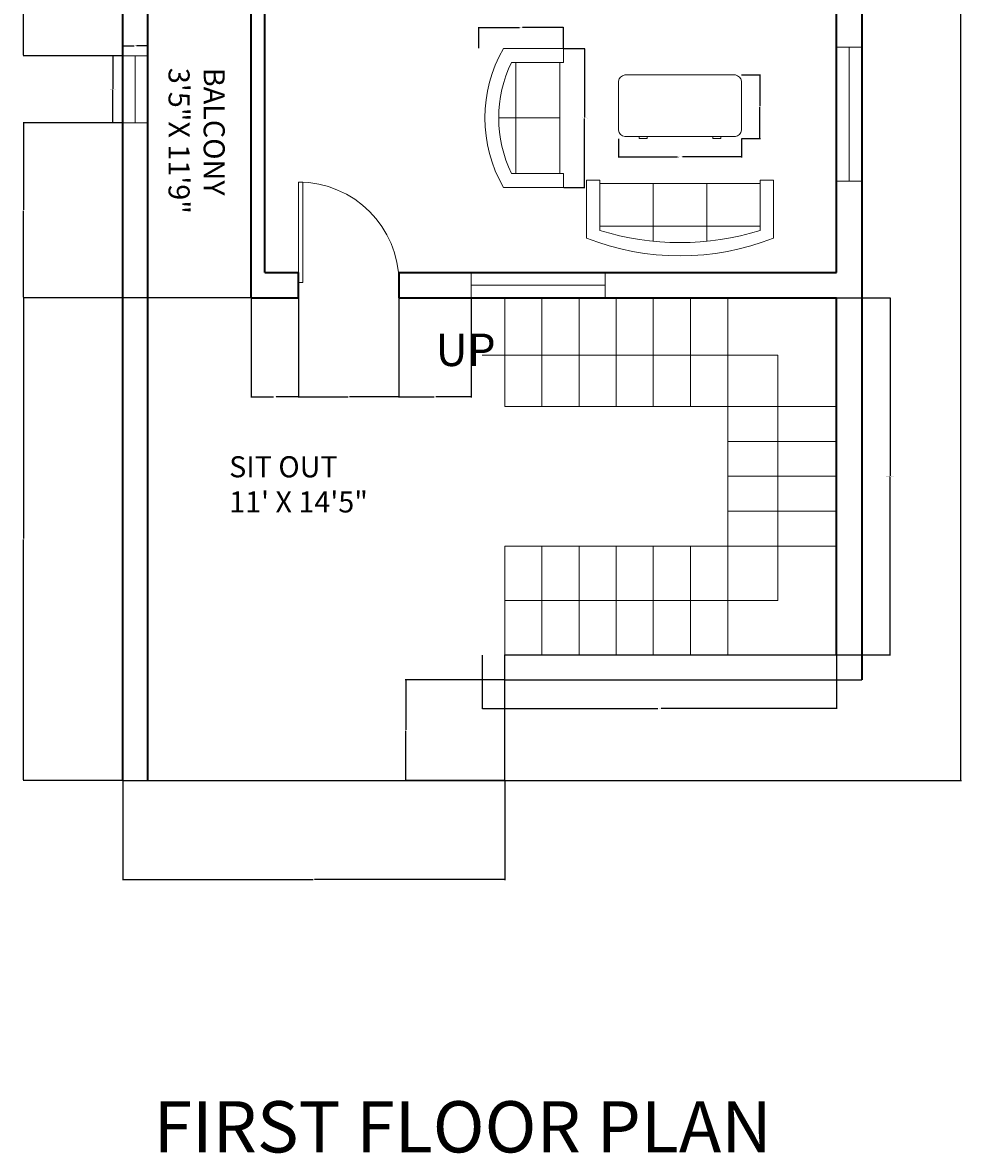
# Model space of a CAD drawing. Units: inches. Extents: x 7766 to 8631, y 9203 to 9940.
# Tile 5 of 6: x 8294 to 8631, y 9203 to 9608. Entities that reach past the tile are written whole.
import ezdxf

# ---------------------------------------------------------------- set-up
doc = ezdxf.new("R2010")
doc.units = ezdxf.units.IN
for name, color, linetype, lineweight in [('A-ANNO-DIMS', 2, 'Continuous', 18), ('A-ANNO-TEXT', 7, 'Continuous', 18), ('A-AREA-IDEN', 11, 'Continuous', 18), ('A-WALL', 7, 'Continuous', 35), ('door', 1, 'Continuous', 18), ('floor', 7, 'Continuous', 25), ('furniture', 6, 'Continuous', 18), ('stair', 2, 'Continuous', 18), ('TITLE', 4, 'Continuous', 35), ('window', 3, 'Continuous', 18)]:
    doc.layers.add(name, color=color, linetype=linetype, lineweight=lineweight)
doc.styles.get("Standard").update_dxf_attribs({"font": 'arial.ttf'})
doc.dimstyles.get("Standard").update_dxf_attribs({"dimtxt": 0.18, "dimasz": 0.18, "dimexe": 0.18, "dimexo": 0.0625, "dimgap": 0.09, "dimtad": 0, "dimtih": 1, "dimtoh": 1, "dimdec": 4, "dimzin": 0, "dimdsep": 46, "dimtxsty": 'Standard', "dimcen": 0.09, "dimadec": 0, "dimazin": 0, "dimtfac": 1, "dimtdec": 4, "dimtofl": 0, "dimtmove": 0, "dimatfit": 3, "dimfxl": 1, "dimtolj": 1, "dimtzin": 0, "dimarcsym": 0})

# ---------------------------------------------------------------- blocks, each defined once
blk = doc.blocks.new('*U2')
for p, q in [((0, 0), (0, -6)), ((40, 0), (40, -6))]:
    blk.add_line(p, q)
blk.add_lwpolyline([(0, 0), (0, 40), (1.75, 40), (1.75, 0)], close=True)
blk.add_arc((0, 0), 40, 0, 90)
blk = doc.blocks.new('Desk - 30 x 60 in.')
for p, q in [((-26.999995, 0), (26.999995, 0)), ((-29.999995, -27), (-29.999995, -3)), ((29.999995, -3), (29.999995, -27)), ((26.999995, -30), (-26.999995, -30)), ((-20.000005, -30), (-20.000005, -31)), ((-20.000005, -31), (-16.000005, -31)), ((-16.000005, -31), (-16.000005, -30)), ((15.999995, -31), (15.999995, -30)), ((19.999995, -31), (15.999995, -31)), ((19.999995, -30), (19.999995, -31))]:
    blk.add_line(p, q)
for centre, start, end in [((-26.499995, -3.5), 98.1301, 171.8699), ((26.499995, -3.5), 8.130102, 81.8699), ((-26.499995, -26.5), 188.1301, 261.8699), ((26.499995, -26.5), 278.1301, 351.8699)]:
    blk.add_arc(centre, 3.535534, start, end)
blk = doc.blocks.new('Sofa - Roundback Loveseat 5 ft.')
for p, q in [((0, -32.44198), (0, -5.99998)), ((-24, -33.99998), (-24, -11.46958)), ((-23.9998, -13.38178), (23.99986, -13.38178)), ((24.00004, -33.99998), (24.00004, -11.46958)), ((-24, -32.44198), (24.00004, -32.44198))]:
    blk.add_line(p, q)
for points in [[(-24, -33.99998), (-30, -33.99998), (-30, -7.99998)], [(30.00004, -7.99998), (30.00004, -33.99998), (24.00004, -33.99998)]]:
    blk.add_lwpolyline(points)
for centre, radius, start, end in [((0, -60.24998), 60.24998, 60.13715, 119.8628), ((0, -61.38438), 55.38444, 64.32083, 115.6792)]:
    blk.add_arc(centre, radius, start, end)
blk = doc.blocks.new('Sofa - Roundback 7 ft.')
for p, q in [((-12.00002, -32.4421), (-12.00003, -6.5971)), ((11.99997, -32.4421), (11.99998, -6.5971)), ((-36.000027, -34), (-36.000027, -11.4696)), ((-35.999844, -13.3819), (35.9998, -13.3819)), ((35.99998, -34), (35.99998, -11.4696)), ((-36.000027, -32.4421), (35.99998, -32.4421))]:
    blk.add_line(p, q)
for points in [[(-36.000027, -34), (-42.000027, -34), (-42.000027, -8)], [(41.99998, -8), (41.99998, -34), (35.99998, -34)]]:
    blk.add_lwpolyline(points)
for centre, radius, start, end in [((0, -114.25), 114.25, 68.43141, 111.5686), ((-0.00001, -127.1968), 121.1968, 72.72033, 107.2797)]:
    blk.add_arc(centre, radius, start, end)
blk = doc.blocks.new('WIN-48IN')
blk.add_line((4.5, 48), (4.5, 0))
blk.add_lwpolyline([(0, 48), (9, 48), (9, 0), (0, 0)], close=True)
blk = doc.blocks.new('WIN-24IN')
blk.add_line((4.5, 24), (4.5, 0))
blk.add_lwpolyline([(0, 24), (9, 24), (9, 0), (0, 0)], close=True)
blk = doc.blocks.new('STAIR-U-RETURN')
for p, q in [((8.13, 89), (8.13, 128)), ((21.45, 89), (21.45, 128)), ((34.76, 89), (34.76, 128)), ((48.08, 89), (48.08, 128)), ((61.39, 89), (61.39, 128)), ((74.71, 89), (74.71, 128)), ((88.13, 0), (88.13, 128)), ((0, 107.36), (106.07, 107.36)), ((106.07, 107.36), (106.07, 19.51)), ((13.13, 89), (8.13, 89)), ((13.13, 89), (88.13, 89)), ((88.13, 89), (127.13, 89)), ((88.13, 76.5), (127.13, 76.5)), ((88.13, 64), (127.13, 64)), ((88.13, 51.5), (127.13, 51.5)), ((8.13, 39), (88.13, 39)), ((8.13, 39), (8.13, 0)), ((21.45, 39), (21.45, 0)), ((34.76, 39), (34.76, 0)), ((48.08, 39), (48.08, 0)), ((61.39, 39), (61.39, 0)), ((74.71, 39), (74.71, 0)), ((88.13, 39), (127.13, 39)), ((106.07, 19.51), (8.13, 19.5))]:
    blk.add_line(p, q)
blk = doc.blocks.new('*D30')
at = {"layer": 'A-ANNO-DIMS', "color": 0, "lineweight": -2, "transparency": 16777216}
for p, q in [((8329.77, 9596.24), (8326.06, 9596.24)), ((8326.24, 9596.06), (8326.24, 9584.42)), ((8326.24, 9572.42), (8326.24, 9584.05)), ((8329.77, 9572.24), (8326.06, 9572.24))]:
    blk.add_line(p, q, dxfattribs=at)
at = {"layer": 'A-ANNO-DIMS', "color": 0, "transparency": 16777216}
for points in [[(8326.21, 9596.06), (8326.27, 9596.06), (8326.24, 9596.24)], [(8326.21, 9572.42), (8326.27, 9572.42), (8326.24, 9572.24)]]:
    blk.add_solid(points, dxfattribs=at)
at = {"layer": 'Defpoints', "color": 0, "transparency": 16777216}
for p in [(8326.24, 9596.24), (8329.84, 9596.24), (8329.84, 9572.24)]:
    blk.add_point(p, dxfattribs=at)
at = {"layer": 'A-ANNO-DIMS', "color": 0, "transparency": 16777216, "insert": (8326.24, 9584.24), "char_height": 0.18, "attachment_point": 5}
blk.add_mtext('\\A1;WINDOW 24 TYP.', dxfattribs=at)
blk = doc.blocks.new('*D31')
at = {"layer": 'A-ANNO-DIMS', "color": 0, "lineweight": -2, "transparency": 16777216}
for p, q in [((8329.84, 9596.3), (8329.84, 9600.02)), ((8330.02, 9599.84), (8333.88, 9599.84)), ((8338.66, 9599.84), (8334.79, 9599.84)), ((8338.84, 9596.3), (8338.84, 9600.02))]:
    blk.add_line(p, q, dxfattribs=at)
at = {"layer": 'A-ANNO-DIMS', "color": 0, "transparency": 16777216}
for points in [[(8330.02, 9599.87), (8330.02, 9599.81), (8329.84, 9599.84)], [(8338.66, 9599.87), (8338.66, 9599.81), (8338.84, 9599.84)]]:
    blk.add_solid(points, dxfattribs=at)
at = {"layer": 'Defpoints', "color": 0, "transparency": 16777216}
for p in [(8338.84, 9599.84), (8329.84, 9596.24), (8338.84, 9596.24)]:
    blk.add_point(p, dxfattribs=at)
at = {"layer": 'A-ANNO-DIMS', "color": 0, "transparency": 16777216, "insert": (8334.34, 9599.84), "char_height": 0.18, "attachment_point": 5}
blk.add_mtext('\\A1;9 TYP.', dxfattribs=at)
blk = doc.blocks.new('*D40')
at = {"layer": 'A-ANNO-DIMS', "color": 0, "lineweight": -2, "transparency": 16777216}
for p, q in [((8507.64, 9566.53), (8507.64, 9559.8)), ((8551.72, 9566.53), (8551.72, 9559.8)), ((8507.82, 9559.98), (8528.78, 9559.98)), ((8551.54, 9559.98), (8530.58, 9559.98))]:
    blk.add_line(p, q, dxfattribs=at)
at = {"layer": 'A-ANNO-DIMS', "color": 0, "transparency": 16777216}
for points in [[(8507.82, 9560.01), (8507.82, 9559.95), (8507.64, 9559.98)], [(8551.54, 9560.01), (8551.54, 9559.95), (8551.72, 9559.98)]]:
    blk.add_solid(points, dxfattribs=at)
at = {"layer": 'Defpoints', "color": 0, "transparency": 16777216}
for p in [(8507.64, 9566.59), (8551.72, 9566.59), (8551.72, 9559.98)]:
    blk.add_point(p, dxfattribs=at)
at = {"layer": 'A-ANNO-DIMS', "color": 0, "transparency": 16777216, "insert": (8529.68, 9559.98), "char_height": 0.18, "attachment_point": 5}
blk.add_mtext('\\A1;DESK 44 TYP.', dxfattribs=at)
blk = doc.blocks.new('*D41')
at = {"layer": 'A-ANNO-DIMS', "color": 0, "lineweight": -2, "transparency": 16777216}
for p, q in [((8551.78, 9589.37), (8558.51, 9589.37)), ((8558.33, 9589.19), (8558.33, 9578.16)), ((8558.33, 9566.77), (8558.33, 9577.8)), ((8551.78, 9566.59), (8558.51, 9566.59))]:
    blk.add_line(p, q, dxfattribs=at)
at = {"layer": 'A-ANNO-DIMS', "color": 0, "transparency": 16777216}
for points in [[(8558.3, 9589.19), (8558.36, 9589.19), (8558.33, 9589.37)], [(8558.3, 9566.77), (8558.36, 9566.77), (8558.33, 9566.59)]]:
    blk.add_solid(points, dxfattribs=at)
at = {"layer": 'Defpoints', "color": 0, "transparency": 16777216}
for p in [(8551.72, 9589.37), (8558.33, 9589.37), (8551.72, 9566.59)]:
    blk.add_point(p, dxfattribs=at)
at = {"layer": 'A-ANNO-DIMS', "color": 0, "transparency": 16777216, "insert": (8558.33, 9577.98), "char_height": 0.18, "attachment_point": 5}
blk.add_mtext('\\A1;23 TYP.', dxfattribs=at)
blk = doc.blocks.new('*D42')
at = {"layer": 'A-ANNO-DIMS', "color": 0, "lineweight": -2, "transparency": 16777216}
for p, q in [((8487.98, 9598.87), (8495.56, 9598.87)), ((8495.38, 9598.69), (8495.38, 9574.16)), ((8495.38, 9549.27), (8495.38, 9573.8)), ((8487.98, 9549.09), (8495.56, 9549.09))]:
    blk.add_line(p, q, dxfattribs=at)
at = {"layer": 'A-ANNO-DIMS', "color": 0, "transparency": 16777216}
for points in [[(8495.35, 9598.69), (8495.41, 9598.69), (8495.38, 9598.87)], [(8495.35, 9549.27), (8495.41, 9549.27), (8495.38, 9549.09)]]:
    blk.add_solid(points, dxfattribs=at)
at = {"layer": 'Defpoints', "color": 0, "transparency": 16777216}
for p in [(8487.91, 9598.87), (8495.38, 9598.87), (8487.91, 9549.09)]:
    blk.add_point(p, dxfattribs=at)
at = {"layer": 'A-ANNO-DIMS', "color": 0, "transparency": 16777216, "insert": (8495.38, 9573.98), "char_height": 0.18, "attachment_point": 5}
blk.add_mtext('\\A1;LOVESEAT 50 TYP.', dxfattribs=at)
blk = doc.blocks.new('*D43')
at = {"layer": 'A-ANNO-DIMS', "color": 0, "lineweight": -2, "transparency": 16777216}
for p, q in [((8457.49, 9598.93), (8457.49, 9606.52)), ((8457.67, 9606.34), (8472.17, 9606.34)), ((8487.73, 9606.34), (8473.23, 9606.34)), ((8487.91, 9598.93), (8487.91, 9606.52))]:
    blk.add_line(p, q, dxfattribs=at)
at = {"layer": 'A-ANNO-DIMS', "color": 0, "transparency": 16777216}
for points in [[(8457.67, 9606.37), (8457.67, 9606.31), (8457.49, 9606.34)], [(8487.73, 9606.37), (8487.73, 9606.31), (8487.91, 9606.34)]]:
    blk.add_solid(points, dxfattribs=at)
at = {"layer": 'Defpoints', "color": 0, "transparency": 16777216}
for p in [(8457.49, 9606.34), (8457.49, 9598.87), (8487.91, 9598.87)]:
    blk.add_point(p, dxfattribs=at)
at = {"layer": 'A-ANNO-DIMS', "color": 0, "transparency": 16777216, "insert": (8472.7, 9606.34), "char_height": 0.18, "attachment_point": 5}
blk.add_mtext('\\A1;30 TYP.', dxfattribs=at)
blk = doc.blocks.new('*D60')
at = {"layer": 'A-ANNO-DIMS', "color": 0, "lineweight": -2, "transparency": 16777216}
for p, q in [((8585.9, 9509.56), (8605.22, 9509.56)), ((8605.04, 9509.38), (8605.04, 9445.75)), ((8605.04, 9381.74), (8605.04, 9445.38)), ((8585.9, 9381.56), (8605.22, 9381.56))]:
    blk.add_line(p, q, dxfattribs=at)
at = {"layer": 'A-ANNO-DIMS', "color": 0, "transparency": 16777216}
for points in [[(8605.01, 9509.38), (8605.07, 9509.38), (8605.04, 9509.56)], [(8605.01, 9381.74), (8605.07, 9381.74), (8605.04, 9381.56)]]:
    blk.add_solid(points, dxfattribs=at)
at = {"layer": 'Defpoints', "color": 0, "transparency": 16777216}
for p in [(8585.84, 9509.56), (8605.04, 9509.56), (8585.84, 9381.56)]:
    blk.add_point(p, dxfattribs=at)
at = {"layer": 'A-ANNO-DIMS', "color": 0, "transparency": 16777216, "insert": (8605.04, 9445.56), "char_height": 0.18, "attachment_point": 5}
blk.add_mtext('\\A1;RETURN STAIR 128 TYP.', dxfattribs=at)
blk = doc.blocks.new('*D61')
at = {"layer": 'A-ANNO-DIMS', "color": 0, "lineweight": -2, "transparency": 16777216}
for p, q in [((8458.7, 9381.5), (8458.7, 9362.18)), ((8585.84, 9381.5), (8585.84, 9362.18)), ((8458.88, 9362.36), (8521.68, 9362.36)), ((8585.66, 9362.36), (8522.86, 9362.36))]:
    blk.add_line(p, q, dxfattribs=at)
at = {"layer": 'A-ANNO-DIMS', "color": 0, "transparency": 16777216}
for points in [[(8458.88, 9362.39), (8458.88, 9362.33), (8458.7, 9362.36)], [(8585.66, 9362.39), (8585.66, 9362.33), (8585.84, 9362.36)]]:
    blk.add_solid(points, dxfattribs=at)
at = {"layer": 'Defpoints', "color": 0, "transparency": 16777216}
for p in [(8458.7, 9381.56), (8585.84, 9381.56), (8585.84, 9362.36)]:
    blk.add_point(p, dxfattribs=at)
at = {"layer": 'A-ANNO-DIMS', "color": 0, "transparency": 16777216, "insert": (8522.27, 9362.36), "char_height": 0.18, "attachment_point": 5}
blk.add_mtext('\\A1;127 TYP.', dxfattribs=at)
blk = doc.blocks.new('*D71')
at = {"layer": 'A-ANNO-DIMS', "color": 0, "lineweight": -2, "transparency": 16777216}
for p, q in [((8594.9, 9904.56), (8630.57, 9904.56)), ((8630.39, 9904.38), (8630.39, 9620.75)), ((8630.39, 9336.74), (8630.39, 9620.38)), ((8466.9, 9336.56), (8630.57, 9336.56))]:
    blk.add_line(p, q, dxfattribs=at)
at = {"layer": 'A-ANNO-DIMS', "color": 0, "transparency": 16777216}
for points in [[(8630.36, 9904.38), (8630.42, 9904.38), (8630.39, 9904.56)], [(8630.36, 9336.74), (8630.42, 9336.74), (8630.39, 9336.56)]]:
    blk.add_solid(points, dxfattribs=at)
at = {"layer": 'Defpoints', "color": 0, "transparency": 16777216}
for p in [(8594.84, 9904.56), (8630.39, 9904.56), (8466.84, 9336.56)]:
    blk.add_point(p, dxfattribs=at)
at = {"layer": 'A-ANNO-DIMS', "color": 0, "transparency": 16777216, "insert": (8630.39, 9620.56), "char_height": 0.18, "attachment_point": 5}
blk.add_mtext('\\A1;568', dxfattribs=at)
blk = doc.blocks.new('*D73')
at = {"layer": 'A-ANNO-DIMS', "color": 0, "lineweight": -2, "transparency": 16777216}
for p, q in [((8329.84, 9336.5), (8329.84, 9300.83)), ((8466.84, 9336.5), (8466.84, 9300.83)), ((8330.02, 9301.01), (8398.06, 9301.01)), ((8466.66, 9301.01), (8398.62, 9301.01))]:
    blk.add_line(p, q, dxfattribs=at)
at = {"layer": 'A-ANNO-DIMS', "color": 0, "transparency": 16777216}
for points in [[(8330.02, 9301.04), (8330.02, 9300.98), (8329.84, 9301.01)], [(8466.66, 9301.04), (8466.66, 9300.98), (8466.84, 9301.01)]]:
    blk.add_solid(points, dxfattribs=at)
at = {"layer": 'Defpoints', "color": 0, "transparency": 16777216}
for p in [(8329.84, 9336.56), (8466.84, 9336.56), (8466.84, 9301.01)]:
    blk.add_point(p, dxfattribs=at)
at = {"layer": 'A-ANNO-DIMS', "color": 0, "transparency": 16777216, "insert": (8398.34, 9301.01), "char_height": 0.18, "attachment_point": 5}
blk.add_mtext('\\A1;137', dxfattribs=at)
blk = doc.blocks.new('*D74')
at = {"layer": 'A-ANNO-DIMS', "color": 0, "lineweight": -2, "transparency": 16777216}
for p, q in [((8375.77, 9509.56), (8294.11, 9509.56)), ((8294.29, 9509.38), (8294.29, 9423.25)), ((8294.29, 9336.74), (8294.29, 9422.88)), ((8329.77, 9336.56), (8294.11, 9336.56))]:
    blk.add_line(p, q, dxfattribs=at)
at = {"layer": 'A-ANNO-DIMS', "color": 0, "transparency": 16777216}
for points in [[(8294.26, 9509.38), (8294.32, 9509.38), (8294.29, 9509.56)], [(8294.26, 9336.74), (8294.32, 9336.74), (8294.29, 9336.56)]]:
    blk.add_solid(points, dxfattribs=at)
at = {"layer": 'Defpoints', "color": 0, "transparency": 16777216}
for p in [(8294.29, 9509.56), (8375.84, 9509.56), (8329.84, 9336.56)]:
    blk.add_point(p, dxfattribs=at)
at = {"layer": 'A-ANNO-DIMS', "color": 0, "transparency": 16777216, "insert": (8294.29, 9423.06), "char_height": 0.18, "attachment_point": 5}
blk.add_mtext('\\A1;173', dxfattribs=at)
blk = doc.blocks.new('*D75')
at = {"layer": 'A-ANNO-DIMS', "color": 0, "lineweight": -2, "transparency": 16777216}
for p, q in [((8466.77, 9372.56), (8431.11, 9372.56)), ((8431.29, 9372.38), (8431.29, 9354.75)), ((8431.29, 9336.74), (8431.29, 9354.38)), ((8466.77, 9336.56), (8431.11, 9336.56))]:
    blk.add_line(p, q, dxfattribs=at)
at = {"layer": 'A-ANNO-DIMS', "color": 0, "transparency": 16777216}
for points in [[(8431.26, 9372.38), (8431.32, 9372.38), (8431.29, 9372.56)], [(8431.26, 9336.74), (8431.32, 9336.74), (8431.29, 9336.56)]]:
    blk.add_solid(points, dxfattribs=at)
at = {"layer": 'Defpoints', "color": 0, "transparency": 16777216}
for p in [(8431.29, 9372.56), (8466.84, 9372.56), (8466.84, 9336.56)]:
    blk.add_point(p, dxfattribs=at)
at = {"layer": 'A-ANNO-DIMS', "color": 0, "transparency": 16777216, "insert": (8431.29, 9354.56), "char_height": 0.18, "attachment_point": 5}
blk.add_mtext('\\A1;36', dxfattribs=at)
blk = doc.blocks.new('*D79')
at = {"layer": 'A-ANNO-DIMS', "color": 0, "lineweight": -2, "transparency": 16777216}
for p, q in [((8329.77, 9698.92), (8294.11, 9698.92)), ((8294.29, 9698.74), (8294.29, 9647.76)), ((8294.29, 9596.42), (8294.29, 9647.4)), ((8329.77, 9596.24), (8294.11, 9596.24))]:
    blk.add_line(p, q, dxfattribs=at)
at = {"layer": 'A-ANNO-DIMS', "color": 0, "transparency": 16777216}
for points in [[(8294.26, 9698.74), (8294.32, 9698.74), (8294.29, 9698.92)], [(8294.26, 9596.42), (8294.32, 9596.42), (8294.29, 9596.24)]]:
    blk.add_solid(points, dxfattribs=at)
at = {"layer": 'Defpoints', "color": 0, "transparency": 16777216}
for p in [(8294.29, 9698.92), (8329.84, 9698.92), (8329.84, 9596.24)]:
    blk.add_point(p, dxfattribs=at)
at = {"layer": 'A-ANNO-DIMS', "color": 0, "transparency": 16777216, "insert": (8294.29, 9647.58), "char_height": 0.18, "attachment_point": 5}
blk.add_mtext('\\A1;102.69', dxfattribs=at)
blk = doc.blocks.new('*D80')
at = {"layer": 'A-ANNO-DIMS', "color": 0, "lineweight": -2, "transparency": 16777216}
for p, q in [((8329.77, 9572.24), (8294.11, 9572.24)), ((8294.29, 9572.06), (8294.29, 9541.08)), ((8294.29, 9509.74), (8294.29, 9540.72)), ((8375.77, 9509.56), (8294.11, 9509.56))]:
    blk.add_line(p, q, dxfattribs=at)
at = {"layer": 'A-ANNO-DIMS', "color": 0, "transparency": 16777216}
for points in [[(8294.26, 9572.06), (8294.32, 9572.06), (8294.29, 9572.24)], [(8294.26, 9509.74), (8294.32, 9509.74), (8294.29, 9509.56)]]:
    blk.add_solid(points, dxfattribs=at)
at = {"layer": 'Defpoints', "color": 0, "transparency": 16777216}
for p in [(8294.29, 9572.24), (8329.84, 9572.24), (8375.84, 9509.56)]:
    blk.add_point(p, dxfattribs=at)
at = {"layer": 'A-ANNO-DIMS', "color": 0, "transparency": 16777216, "insert": (8294.29, 9540.9), "char_height": 0.18, "attachment_point": 5}
blk.add_mtext('\\A1;62.67', dxfattribs=at)
blk = doc.blocks.new('*D87')
at = {"layer": 'A-ANNO-DIMS', "color": 0, "lineweight": -2, "transparency": 16777216}
for p, q in [((8392.89, 9509.5), (8392.89, 9473.83)), ((8428.89, 9509.5), (8428.89, 9473.83)), ((8393.07, 9474.01), (8410.67, 9474.01)), ((8428.71, 9474.01), (8411.11, 9474.01))]:
    blk.add_line(p, q, dxfattribs=at)
at = {"layer": 'A-ANNO-DIMS', "color": 0, "transparency": 16777216}
for points in [[(8393.07, 9474.04), (8393.07, 9473.98), (8392.89, 9474.01)], [(8428.71, 9474.04), (8428.71, 9473.98), (8428.89, 9474.01)]]:
    blk.add_solid(points, dxfattribs=at)
at = {"layer": 'Defpoints', "color": 0, "transparency": 16777216}
for p in [(8392.89, 9509.56), (8428.89, 9509.56), (8392.89, 9474.01)]:
    blk.add_point(p, dxfattribs=at)
at = {"layer": 'A-ANNO-DIMS', "color": 0, "transparency": 16777216, "insert": (8410.89, 9474.01), "char_height": 0.18, "attachment_point": 5}
blk.add_mtext('\\A1;36', dxfattribs=at)
blk = doc.blocks.new('*D88')
at = {"layer": 'A-ANNO-DIMS', "color": 0, "lineweight": -2, "transparency": 16777216}
for p, q in [((8428.89, 9509.5), (8428.89, 9473.83)), ((8454.79, 9509.5), (8454.79, 9473.83)), ((8429.07, 9474.01), (8441.51, 9474.01)), ((8454.61, 9474.01), (8442.16, 9474.01))]:
    blk.add_line(p, q, dxfattribs=at)
at = {"layer": 'A-ANNO-DIMS', "color": 0, "transparency": 16777216}
for points in [[(8429.07, 9474.04), (8429.07, 9473.98), (8428.89, 9474.01)], [(8454.61, 9474.04), (8454.61, 9473.98), (8454.79, 9474.01)]]:
    blk.add_solid(points, dxfattribs=at)
at = {"layer": 'Defpoints', "color": 0, "transparency": 16777216}
for p in [(8428.89, 9509.56), (8454.79, 9509.56), (8428.89, 9474.01)]:
    blk.add_point(p, dxfattribs=at)
at = {"layer": 'A-ANNO-DIMS', "color": 0, "transparency": 16777216, "insert": (8441.84, 9474.01), "char_height": 0.18, "attachment_point": 5}
blk.add_mtext('\\A1;25.9', dxfattribs=at)
blk = doc.blocks.new('*D89')
at = {"layer": 'A-ANNO-DIMS', "color": 0, "lineweight": -2, "transparency": 16777216}
for p, q in [((8375.84, 9509.5), (8375.84, 9473.83)), ((8392.89, 9509.5), (8392.89, 9473.83)), ((8376.02, 9474.01), (8383.91, 9474.01)), ((8392.71, 9474.01), (8384.82, 9474.01))]:
    blk.add_line(p, q, dxfattribs=at)
at = {"layer": 'A-ANNO-DIMS', "color": 0, "transparency": 16777216}
for points in [[(8376.02, 9474.04), (8376.02, 9473.98), (8375.84, 9474.01)], [(8392.71, 9474.04), (8392.71, 9473.98), (8392.89, 9474.01)]]:
    blk.add_solid(points, dxfattribs=at)
at = {"layer": 'Defpoints', "color": 0, "transparency": 16777216}
for p in [(8375.84, 9509.56), (8392.89, 9509.56), (8375.84, 9474.01)]:
    blk.add_point(p, dxfattribs=at)
at = {"layer": 'A-ANNO-DIMS', "color": 0, "transparency": 16777216, "insert": (8384.36, 9474.01), "char_height": 0.18, "attachment_point": 5}
blk.add_mtext('\\A1;17.052', dxfattribs=at)

msp = doc.modelspace()

# ---------------------------------------------------------------- linework, layer by layer
at = {"layer": 'A-WALL'}
for p, q in [((8329.8366, 9336.5631), (8329.8366, 9904.5631)), ((8338.8366, 9509.5631), (8338.8366, 9895.5631)), ((8594.8366, 9895.5631), (8594.8366, 9372.5631)), ((8375.8366, 9509.5631), (8375.8366, 9665.3613)), ((8380.8366, 9518.5631), (8380.8366, 9665.3613)), ((8585.8366, 9518.5631), (8585.8366, 9650.5631)), ((8380.8366, 9518.5631), (8392.8883, 9518.5631)), ((8428.8883, 9518.5631), (8437.8366, 9518.5631)), ((8428.8883, 9518.5631), (8453.7386, 9518.5631)), ((8442.8366, 9518.5631), (8471.8366, 9518.5631)), ((8466.8366, 9518.5631), (8471.8366, 9518.5631)), ((8471.8366, 9518.5631), (8585.8366, 9518.5631)), ((8338.8366, 9336.5631), (8338.8366, 9509.5631)), ((8375.8366, 9509.5631), (8392.8883, 9509.5631)), ((8428.8883, 9509.5631), (8471.8366, 9509.5631)), ((8466.8366, 9509.5631), (8471.8366, 9509.5631)), ((8471.8366, 9509.5631), (8585.8366, 9509.5631)), ((8585.8366, 9381.5631), (8585.8366, 9509.5631))]:
    msp.add_line(p, q, dxfattribs=at)
for points in [[(8392.8883, 9509.5631), (8392.8883, 9518.5631)], [(8428.8883, 9518.5631), (8428.8883, 9509.5631)]]:
    msp.add_lwpolyline(points, dxfattribs=at)
at = {"layer": 'floor'}
for p, q in [((8466.8366, 9381.5631), (8594.8366, 9381.5631)), ((8466.8366, 9372.5631), (8466.8366, 9381.5631)), ((8466.8366, 9372.5631), (8585.8366, 9372.5631)), ((8466.8366, 9336.5631), (8466.8366, 9372.5631)), ((8585.8366, 9372.5631), (8594.8366, 9372.5631)), ((8329.8366, 9336.5631), (8392.8883, 9336.5631)), ((8338.8366, 9336.5631), (8466.8366, 9336.5631))]:
    msp.add_line(p, q, dxfattribs=at)
msp.add_lwpolyline([(8466.8366, 9336.5631), (8466.8366, 9372.5631), (8585.8366, 9372.5631)], dxfattribs=at)

# ---------------------------------------------------------------- block references
at = {"layer": 'door', "xscale": 0.9, "yscale": 0.9, "zscale": 0.9}
msp.add_blockref('*U2', (8392.8883, 9514.9631), dxfattribs=at)
at = {"layer": 'furniture'}
for name, p, xscale, yscale, zscale, rotation in [('Sofa - Roundback Loveseat 5 ft.', (8459.7024, 9573.9784), 0.829764444386874, 0.829764444386874, 0.829764444386874, 90), ('Sofa - Roundback 7 ft.', (8529.6811, 9524.5295), 0.7986556834992792, 0.7986556834992792, 0.7986556834992792, 180)]:
    msp.add_blockref(name, p, dxfattribs=dict(at, xscale=xscale, yscale=yscale, zscale=zscale, rotation=rotation))
at = {"layer": 'furniture', "xscale": 0.7346827235755428, "yscale": 0.7346827235755428, "zscale": 0.7346827235755428}
msp.add_blockref('Desk - 30 x 60 in.', (8529.6811, 9589.3674), dxfattribs=at)
at = {"layer": 'stair'}
msp.add_blockref('STAIR-U-RETURN', (8458.7036, 9381.563), dxfattribs=at)
at = {"layer": 'window'}
for name, p in [('WIN-24IN', (8329.8366, 9572.2351)), ('WIN-48IN', (8585.8366, 9551.2965))]:
    msp.add_blockref(name, p, dxfattribs=at)
at = {"layer": 'window', "rotation": 89.99999999999817}
msp.add_blockref('WIN-48IN', (8502.7899, 9509.5631), dxfattribs=at)

# ---------------------------------------------------------------- texts
at = {"layer": 'A-ANNO-TEXT'}
msp.add_text('UP', height=11.64486, dxfattribs=at).set_placement((8442.0447, 9485.0619))
at = {"layer": 'A-AREA-IDEN', "insert": (8366.4068, 9591.9215), "char_height": 7.556341, "attachment_point": 1, "rotation": 270}
msp.add_mtext_dynamic_manual_height_columns('BALCONY\\P3\'5"X 11\'9"', width=97.347002, gutter_width=18.8909, heights=[0], dxfattribs=at)
at = {"layer": 'A-AREA-IDEN', "insert": (8367.9856, 9452.7426), "char_height": 7.556341, "attachment_point": 1}
msp.add_mtext_dynamic_manual_height_columns('SIT OUT\\P11\' X 14\'5"', width=97.347002, gutter_width=18.8909, heights=[0], dxfattribs=at)
at = {"layer": 'TITLE'}
msp.add_text('FIRST FLOOR PLAN', height=18.381464, dxfattribs=at).set_placement((8340.8374, 9203.2441))

# ---------------------------------------------------------------- dimensions: what is measured, and where the dimension line sits
at = {"layer": 'A-ANNO-DIMS'}
for base, p1, p2, angle, override, picture, middle in [((8630.3866, 9904.5631), (8466.8366, 9336.5631), (8594.8366, 9904.5631), 90, {"dimdec": 0, "dimlfac": 1, "dimrnd": 0, "dimzin": 0, "dimdsep": 46, "dimlunit": 2}, '*D71', (8630.3866, 9620.5631)), ((8294.2866, 9698.9207), (8329.8366, 9596.2356), (8329.8366, 9698.9207), 90, {"dimdec": 2, "dimlfac": 1, "dimrnd": 0, "dimzin": 0, "dimdsep": 46, "dimlunit": 2}, '*D79', (8294.2866, 9647.5781)), ((8294.2866, 9572.2356), (8375.8366, 9509.5631), (8329.8366, 9572.2356), 90, {"dimdec": 2, "dimlfac": 1, "dimrnd": 0, "dimzin": 0, "dimdsep": 46, "dimlunit": 2}, '*D80', (8294.2866, 9540.8993)), ((8294.2866, 9509.5631), (8329.8366, 9336.5631), (8375.8366, 9509.5631), 90, {"dimdec": 0, "dimlfac": 1, "dimrnd": 0, "dimzin": 0, "dimdsep": 46, "dimlunit": 2}, '*D74', (8294.2866, 9423.0631)), ((8375.8366, 9474.0131), (8392.8883, 9509.5631), (8375.8366, 9509.5631), 180, {"dimdec": 3, "dimlfac": 1, "dimrnd": 0, "dimzin": 0, "dimdsep": 46, "dimlunit": 2}, '*D89', (8384.3624, 9474.0131)), ((8392.8883, 9474.0131), (8428.8883, 9509.5631), (8392.8883, 9509.5631), 180, {"dimdec": 0, "dimlfac": 1, "dimrnd": 0, "dimzin": 0, "dimdsep": 46, "dimlunit": 2}, '*D87', (8410.8883, 9474.0131)), ((8428.8883, 9474.0131), (8454.7902, 9509.5631), (8428.8883, 9509.5631), 180, {"dimdec": 1, "dimlfac": 1, "dimrnd": 0, "dimzin": 0, "dimdsep": 46, "dimlunit": 2}, '*D88', (8441.8393, 9474.0131)), ((8431.2866, 9372.5631), (8466.8366, 9336.5631), (8466.8366, 9372.5631), 90, {"dimdec": 0, "dimlfac": 1, "dimrnd": 0, "dimzin": 0, "dimdsep": 46, "dimlunit": 2}, '*D75', (8431.2866, 9354.5631))]:
    dim = msp.add_linear_dim(base=base, p1=p1, p2=p2, angle=angle, dimstyle='Standard', override=override, dxfattribs=at)
    dim.commit()
    dim.dimension.update_dxf_attribs({"geometry": picture, "text_midpoint": middle})
for base, p1, p2, angle, text, picture, middle in [((8457.4897, 9606.3392), (8487.9144, 9598.8713), (8457.4897, 9598.8713), 180, '<> TYP.', '*D43', (8472.702, 9606.3392)), ((8326.2366, 9596.2356), (8329.8366, 9572.2356), (8329.8366, 9596.2356), 90, 'WINDOW <> TYP.', '*D30', (8326.2366, 9584.2356)), ((8495.3822, 9598.8713), (8487.9144, 9549.0854), (8487.9144, 9598.8713), 90, 'LOVESEAT <> TYP.', '*D42', (8495.3822, 9573.9784)), ((8558.3338, 9589.3674), (8551.7216, 9566.5922), (8551.7216, 9589.3674), 90, '<> TYP.', '*D41', (8558.3338, 9577.9798)), ((8605.0366, 9509.5631), (8585.8366, 9381.5631), (8585.8366, 9509.5631), 90, 'RETURN STAIR <> TYP.', '*D60', (8605.0366, 9445.5631))]:
    dim = msp.add_linear_dim(base=base, p1=p1, p2=p2, angle=angle, text=text, dimstyle='Standard', override={"dimdec": 0, "dimlfac": 1, "dimrnd": 0, "dimzin": 0, "dimdsep": 46, "dimlunit": 2}, dxfattribs=at)
    dim.commit()
    dim.dimension.update_dxf_attribs({"geometry": picture, "text_midpoint": middle})
for base, p1, p2, text, picture, middle in [((8338.8366, 9599.8356), (8329.8366, 9596.2356), (8338.8366, 9596.2356), '<> TYP.', '*D31', (8334.3366, 9599.8356)), ((8551.7216, 9559.9801), (8507.6407, 9566.5922), (8551.7216, 9566.5922), 'DESK <> TYP.', '*D40', (8529.6811, 9559.9801)), ((8585.8366, 9362.3631), (8458.704, 9381.5631), (8585.8366, 9381.5631), '<> TYP.', '*D61', (8522.2703, 9362.3631))]:
    dim = msp.add_linear_dim(base=base, p1=p1, p2=p2, text=text, dimstyle='Standard', override={"dimdec": 0, "dimlfac": 1, "dimrnd": 0, "dimzin": 0, "dimdsep": 46, "dimlunit": 2}, dxfattribs=at)
    dim.commit()
    dim.dimension.update_dxf_attribs({"geometry": picture, "text_midpoint": middle})
dim = msp.add_linear_dim(base=(8466.8366, 9301.0131), p1=(8329.8366, 9336.5631), p2=(8466.8366, 9336.5631), dimstyle='Standard', override={"dimdec": 0, "dimlfac": 1, "dimrnd": 0, "dimzin": 0, "dimdsep": 46, "dimlunit": 2}, dxfattribs=at)
dim.commit()
dim.dimension.update_dxf_attribs({"geometry": '*D73', "text_midpoint": (8398.3366, 9301.0131)})

doc.saveas('drawing.dxf')
